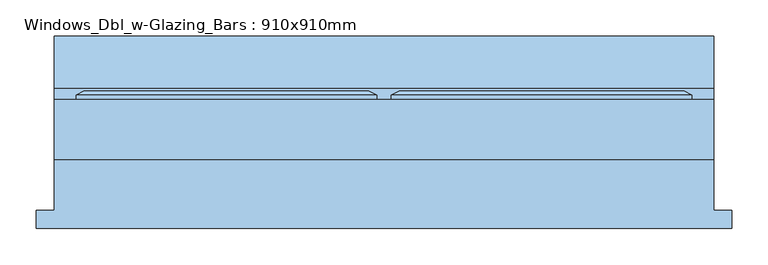
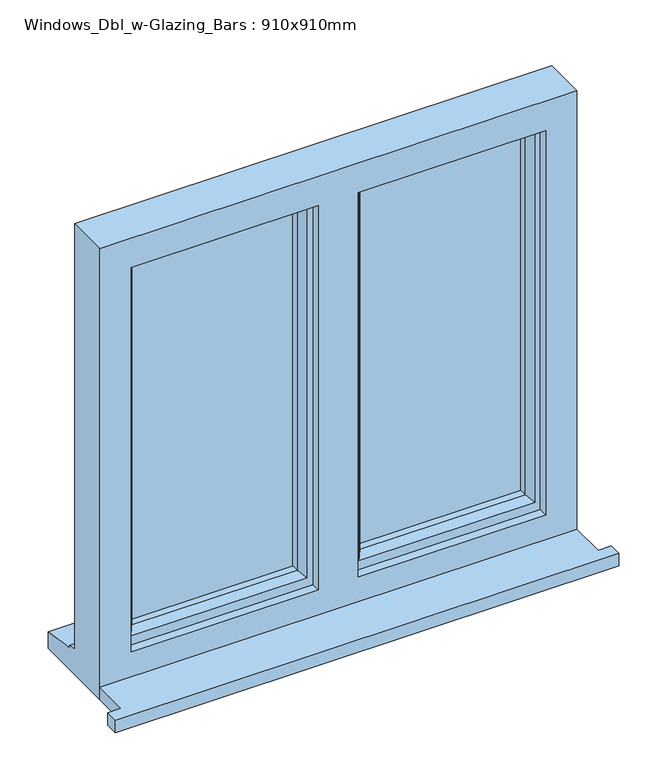
"""IFC4 building model written with IfcOpenShell, lengths in millimetres: window geometry, Windows_Dbl_w-Glazing_Bars : 910x910mm."""

from ifc_helpers import new_model, si_unit, frame, origin, place, context, project, spatial, polyline, outline, extrude, faceted_brep, source, transform, mapped, element, save


def windows_dbl_w_glazing_bars_910x910mm_41eba874(model_context):
    return source(origin(), model_context, "Body", "SolidModel", [
        extrude(outline(polyline([(-610.0, -118.1434322), (-610.0, -93.1434322), (-585.0, -93.1434322), (-585.0, -22.9434322), (325.0, -22.9434322), (325.0, -93.1434322), (350.0, -93.1434322), (350.0, -118.1434322), (-610.0, -118.1434322)])), frame((0.0, 0.0, 1190.0), z_axis=(0.0, 0.0, 1.0), x_axis=(1.0, 0.0, 0.0)), (0.0, 0.0, 1.0), 25.0),
        faceted_brep([(-120.0, 60.0565678, 2070.0), (-120.0, 65.8300705, 2070.0), (-120.0, 65.8300705, 1243.0), (-120.0, 60.0565678, 1243.0), (-110.0, -4.9434322, 2060.0), (-110.0, 60.0565678, 2060.0), (-110.0, 60.0565678, 1253.0), (-110.0, -4.9434322, 1253.0), (-70.0, 9.5494677, 2020.0), (-80.1480377, -4.9434322, 2030.1480377), (-80.1480377, -4.9434322, 1282.8519623), (-70.0, 9.5494677, 1293.0), (-70.0, 24.0565678, 2020.0), (-70.0, 24.0565678, 1293.0), (-80.0, 48.0565678, 2030.0), (-80.0, 24.0565678, 2030.0), (-80.0, 24.0565678, 1283.0), (-80.0, 48.0565678, 1283.0), (-70.0, 65.8300705, 2020.0), (-70.0, 48.0565678, 2020.0), (-70.0, 48.0565678, 1293.0), (-70.0, 65.8300705, 1293.0), (-87.4457548, 71.6035732, 2037.4457548), (-87.4457548, 71.6035732, 1275.5542452), (-109.2153903, 71.6035732, 2059.2153903), (-109.2153903, 71.6035732, 1253.7846097), (295.0, 65.8300705, 1243.0), (295.0, 60.0565678, 1243.0), (285.0, 60.0565678, 1253.0), (285.0, -4.9434322, 1253.0), (255.1480377, -4.9434322, 1282.8519623), (245.0, 9.5494677, 1293.0), (245.0, 24.0565678, 1293.0), (255.0, 24.0565678, 1283.0), (255.0, 48.0565678, 1283.0), (245.0, 48.0565678, 1293.0), (245.0, 65.8300705, 1293.0), (262.4457548, 71.6035732, 1275.5542452), (284.2153903, 71.6035732, 1253.7846097), (295.0, 65.8300705, 2070.0), (295.0, 60.0565678, 2070.0), (285.0, 60.0565678, 2060.0), (285.0, -4.9434322, 2060.0), (255.1480377, -4.9434322, 2030.1480377), (245.0, 9.5494677, 2020.0), (245.0, 24.0565678, 2020.0), (255.0, 24.0565678, 2030.0), (255.0, 48.0565678, 2030.0), (245.0, 48.0565678, 2020.0), (245.0, 65.8300705, 2020.0), (262.4457548, 71.6035732, 2037.4457548), (284.2153903, 71.6035732, 2059.2153903)], [[[0, 1, 2, 3]], [[4, 5, 6, 7]], [[8, 9, 10, 11]], [[12, 8, 11, 13]], [[14, 15, 16, 17]], [[18, 19, 20, 21]], [[22, 18, 21, 23]], [[1, 24, 25, 2]], [[3, 2, 26, 27]], [[7, 6, 28, 29]], [[11, 10, 30, 31]], [[13, 11, 31, 32]], [[17, 16, 33, 34]], [[21, 20, 35, 36]], [[23, 21, 36, 37]], [[2, 25, 38, 26]], [[27, 26, 39, 40]], [[29, 28, 41, 42]], [[31, 30, 43, 44]], [[32, 31, 44, 45]], [[34, 33, 46, 47]], [[36, 35, 48, 49]], [[37, 36, 49, 50]], [[26, 38, 51, 39]], [[40, 39, 1, 0]], [[3, 27, 40, 0], [5, 41, 28, 6]], [[42, 41, 5, 4]], [[7, 29, 42, 4], [9, 43, 30, 10]], [[44, 43, 9, 8]], [[45, 44, 8, 12]], [[15, 46, 33, 16], [13, 32, 45, 12]], [[47, 46, 15, 14]], [[17, 34, 47, 14], [19, 48, 35, 20]], [[49, 48, 19, 18]], [[50, 49, 18, 22]], [[24, 51, 38, 25], [23, 37, 50, 22]], [[39, 51, 24, 1]]]),
        extrude(outline(polyline([(255.0, 24.0565678), (-80.0, 24.0565678), (-80.0, 48.0565678), (255.0, 48.0565678), (255.0, 24.0565678)])), frame((0.0, 0.0, 1283.0), z_axis=(0.0, 0.0, 1.0), x_axis=(1.0, 0.0, 0.0)), (0.0, 0.0, 1.0), 747.0),
        extrude(outline(polyline([(-180.0, 24.0565678), (-515.0, 24.0565678), (-515.0, 48.0565678), (-180.0, 48.0565678), (-180.0, 24.0565678)])), frame((0.0, 0.0, 1283.0), z_axis=(0.0, 0.0, 1.0), x_axis=(1.0, 0.0, 0.0)), (0.0, 0.0, 1.0), 747.0),
        faceted_brep([(-140.0, 60.0565678, 2070.0), (-140.0, 65.8300705, 2070.0), (-555.0, 65.8300705, 2070.0), (-555.0, 60.0565678, 2070.0), (-150.0, -4.9434322, 2060.0), (-150.0, 60.0565678, 2060.0), (-545.0, 60.0565678, 2060.0), (-545.0, -4.9434322, 2060.0), (-190.0, 9.5494677, 2020.0), (-179.8519623, -4.9434322, 2030.1480377), (-515.1480377, -4.9434322, 2030.1480377), (-505.0, 9.5494677, 2020.0), (-190.0, 24.0565678, 2020.0), (-505.0, 24.0565678, 2020.0), (-180.0, 48.0565678, 2030.0), (-180.0, 24.0565678, 2030.0), (-515.0, 24.0565678, 2030.0), (-515.0, 48.0565678, 2030.0), (-190.0, 65.8300705, 2020.0), (-190.0, 48.0565678, 2020.0), (-505.0, 48.0565678, 2020.0), (-505.0, 65.8300705, 2020.0), (-172.5542452, 71.6035732, 2037.4457548), (-522.4457548, 71.6035732, 2037.4457548), (-150.7846097, 71.6035732, 2059.2153903), (-544.2153903, 71.6035732, 2059.2153903), (-555.0, 65.8300705, 1243.0), (-555.0, 60.0565678, 1243.0), (-545.0, 60.0565678, 1253.0), (-545.0, -4.9434322, 1253.0), (-515.1480377, -4.9434322, 1282.8519623), (-505.0, 9.5494677, 1293.0), (-505.0, 24.0565678, 1293.0), (-515.0, 24.0565678, 1283.0), (-515.0, 48.0565678, 1283.0), (-505.0, 48.0565678, 1293.0), (-505.0, 65.8300705, 1293.0), (-522.4457548, 71.6035732, 1275.5542452), (-544.2153903, 71.6035732, 1253.7846097), (-140.0, 65.8300705, 1243.0), (-140.0, 60.0565678, 1243.0), (-150.0, 60.0565678, 1253.0), (-150.0, -4.9434322, 1253.0), (-179.8519623, -4.9434322, 1282.8519623), (-190.0, 9.5494677, 1293.0), (-190.0, 24.0565678, 1293.0), (-180.0, 24.0565678, 1283.0), (-180.0, 48.0565678, 1283.0), (-190.0, 48.0565678, 1293.0), (-190.0, 65.8300705, 1293.0), (-172.5542452, 71.6035732, 1275.5542452), (-150.7846097, 71.6035732, 1253.7846097)], [[[0, 1, 2, 3]], [[4, 5, 6, 7]], [[8, 9, 10, 11]], [[12, 8, 11, 13]], [[14, 15, 16, 17]], [[18, 19, 20, 21]], [[22, 18, 21, 23]], [[1, 24, 25, 2]], [[3, 2, 26, 27]], [[7, 6, 28, 29]], [[11, 10, 30, 31]], [[13, 11, 31, 32]], [[17, 16, 33, 34]], [[21, 20, 35, 36]], [[23, 21, 36, 37]], [[2, 25, 38, 26]], [[27, 26, 39, 40]], [[0, 3, 27, 40], [41, 28, 6, 5]], [[29, 28, 41, 42]], [[4, 7, 29, 42], [43, 30, 10, 9]], [[31, 30, 43, 44]], [[32, 31, 44, 45]], [[46, 33, 16, 15], [12, 13, 32, 45]], [[34, 33, 46, 47]], [[14, 17, 34, 47], [48, 35, 20, 19]], [[36, 35, 48, 49]], [[37, 36, 49, 50]], [[51, 38, 25, 24], [22, 23, 37, 50]], [[26, 38, 51, 39]], [[40, 39, 1, 0]], [[42, 41, 5, 4]], [[44, 43, 9, 8]], [[45, 44, 8, 12]], [[47, 46, 15, 14]], [[49, 48, 19, 18]], [[50, 49, 18, 22]], [[39, 51, 24, 1]]]),
        extrude(outline(polyline([(-80.1480377, 40.0565678), (255.0, 40.0565678), (255.0, 32.0565678), (-80.1480377, 32.0565678), (-80.1480377, 40.0565678)])), frame((0.0, 0.0, 1646.5), z_axis=(0.0, 0.0, 1.0), x_axis=(1.0, 0.0, 0.0)), (0.0, 0.0, 1.0), 20.0),
        extrude(outline(polyline([(-515.0, 40.0565678), (-180.0, 40.0565678), (-180.0, 32.0565678), (-515.0, 32.0565678), (-515.0, 40.0565678)])), frame((0.0, 0.0, 1646.5), z_axis=(0.0, 0.0, 1.0), x_axis=(1.0, 0.0, 0.0)), (0.0, 0.0, 1.0), 20.0),
        extrude(outline(polyline([(-80.1480377, 40.0565678), (255.0, 40.0565678), (255.0, 32.0565678), (-80.1480377, 32.0565678), (-80.1480377, 40.0565678)])), frame((0.0, 0.0, 1828.25), z_axis=(0.0, 0.0, 1.0), x_axis=(1.0, 0.0, 0.0)), (0.0, 0.0, 1.0), 20.0),
        extrude(outline(polyline([(-80.1480377, 40.0565678), (255.0, 40.0565678), (255.0, 32.0565678), (-80.1480377, 32.0565678), (-80.1480377, 40.0565678)])), frame((0.0, 0.0, 1464.75), z_axis=(0.0, 0.0, 1.0), x_axis=(1.0, 0.0, 0.0)), (0.0, 0.0, 1.0), 20.0),
        extrude(outline(polyline([(-515.0, 40.0565678), (-180.0, 40.0565678), (-180.0, 32.0565678), (-515.0, 32.0565678), (-515.0, 40.0565678)])), frame((0.0, 0.0, 1828.25), z_axis=(0.0, 0.0, 1.0), x_axis=(1.0, 0.0, 0.0)), (0.0, 0.0, 1.0), 20.0),
        extrude(outline(polyline([(-515.0, 40.0565678), (-180.0, 40.0565678), (-180.0, 32.0565678), (-515.0, 32.0565678), (-515.0, 40.0565678)])), frame((0.0, 0.0, 1464.75), z_axis=(0.0, 0.0, 1.0), x_axis=(1.0, 0.0, 0.0)), (0.0, 0.0, 1.0), 20.0),
        faceted_brep([(325.0, -22.9434322, 2100.0), (-585.0, -22.9434322, 2100.0), (-585.0, -22.9434322, 1190.0), (325.0, -22.9434322, 1190.0), (265.0, -22.9434322, 2040.0), (265.0, -22.9434322, 1265.0), (-92.0, -22.9434322, 1265.0), (-92.0, -22.9434322, 2040.0), (-168.0, -22.9434322, 2040.0), (-168.0, -22.9434322, 1265.0), (-525.0, -22.9434322, 1265.0), (-525.0, -22.9434322, 2040.0), (-585.0, 60.0565678, 2100.0), (-585.0, 60.0565678, 1241.0), (-585.0, 75.0565678, 1239.68767), (-585.0, 75.0565678, 1234.7449676), (-585.0, 147.5565678, 1223.8088847), (-585.0, 147.5565678, 1190.0), (325.0, 60.0565678, 2100.0), (325.0, 60.0565678, 1241.0), (-545.0, 60.0565678, 2060.0), (-545.0, 60.0565678, 1253.0), (-150.0, 60.0565678, 1253.0), (-150.0, 60.0565678, 2060.0), (-110.0, 60.0565678, 2060.0), (-110.0, 60.0565678, 1253.0), (285.0, 60.0565678, 1253.0), (285.0, 60.0565678, 2060.0), (-545.0, -4.9434322, 2060.0), (-545.0, -4.9434322, 1253.0), (-150.0, -4.9434322, 2060.0), (-150.0, -4.9434322, 1253.0), (-168.0, -4.9434322, 2040.0), (-525.0, -4.9434322, 2040.0), (-525.0, -4.9434322, 1265.0), (-168.0, -4.9434322, 1265.0), (-110.0, -4.9434322, 2060.0), (285.0, -4.9434322, 2060.0), (285.0, -4.9434322, 1253.0), (-110.0, -4.9434322, 1253.0), (265.0, -4.9434322, 2040.0), (-92.0, -4.9434322, 2040.0), (-92.0, -4.9434322, 1265.0), (265.0, -4.9434322, 1265.0), (325.0, 147.5565678, 1190.0), (325.0, 147.5565678, 1223.8088847), (325.0, 75.0565678, 1234.7449676), (325.0, 75.0565678, 1239.68767)], [[[0, 1, 2, 3], [4, 5, 6, 7], [8, 9, 10, 11]], [[2, 1, 12, 13, 14, 15, 16, 17]], [[13, 12, 18, 19], [20, 21, 22, 23], [24, 25, 26, 27]], [[21, 20, 28, 29]], [[28, 30, 31, 29], [32, 33, 34, 35]], [[36, 37, 38, 39], [40, 41, 42, 43]], [[33, 11, 10, 34]], [[1, 0, 18, 12]], [[28, 20, 23, 30]], [[27, 37, 36, 24]], [[11, 33, 32, 8]], [[40, 4, 7, 41]], [[19, 18, 0, 3, 44, 45, 46, 47]], [[27, 26, 38, 37]], [[4, 40, 43, 5]], [[41, 7, 6, 42]], [[8, 32, 35, 9]], [[23, 22, 31, 30]], [[25, 24, 36, 39]], [[44, 3, 2, 17]], [[45, 44, 17, 16]], [[46, 45, 16, 15]], [[47, 46, 15, 14]], [[19, 47, 14, 13]], [[22, 21, 29, 31]], [[39, 38, 26, 25]], [[6, 5, 43, 42]], [[35, 34, 10, 9]]]),
    ])


if __name__ == "__main__":
    model = new_model("IFC4")
    model_context = context("Model", 3, world=origin())
    ifc_project = project(units=[si_unit("LENGTHUNIT", "METRE", prefix="MILLI")], contexts=[model_context])
    site = spatial("IfcSite", under=ifc_project)
    building = spatial("IfcBuilding", under=site)
    placement = place(None, origin())
    windows_dbl_w_glazing_bars_910x910mm_shape = windows_dbl_w_glazing_bars_910x910mm_41eba874(model_context)
    element("IfcWindow", 1, ObjectType="Windows_Dbl_w-Glazing_Bars : 910x910mm", at=placement, inside=building, context=model_context, shape_type="MappedRepresentation", body=[
        mapped(windows_dbl_w_glazing_bars_910x910mm_shape, transform((0.0, 0.0, 0.0), x_axis=(1.0, 0.0, 0.0), y_axis=(0.0, 1.0, 0.0), z_axis=(0.0, 0.0, 1.0))),
    ])
    save(model, "model.ifc")

# Revit data of these elements
# Type "Windows_Dbl_w-Glazing_Bars : 910x910mm"
#   Type Mark = "33"
#   Operation = "DoublePanelVertical"
#   Construction Type Id = "GSP4R"
#   Manufacturer = "Revit"
#   Keynote = "L10"
#   Analytic Construction = "1/8 in Pilkington single glazing"
#   Wrap Layers (Ext) from Ext = 0' - 4.03543"
#   Wrap Layers (Int) from Ext = 0' - 6.98819"
#   Window Board Projection = 0' - 0.98425"
#   Window Board Extension = 0' - 0.98425"
#   Visual Light Transmittance = 0.9
#   Solar Heat Gain Coefficient = 0.78
#   Rough Width = 2' - 11.82677"
#   Rough Height = 2' - 11.82677"
#   Height = 2' - 11.82677"
#   Width = 2' - 11.82677"
#   Heat Transfer Coefficient (U) = 0.6496 BTU/(h·ft²·°F)
#   Glazing Thickness = 0' - 0.94488"
#   Glazing Bar Thickness = 0' - 0.7874"
#   FrameOffset - External = 0' - 1.9685"
#   Frame Depth = 0' - 2.55906"
#   Default Head Height = 6' - 10.67717"
#   Cill Depth = 0' - 3.44488"
#   Cavity Closer Width = 0' - 1.9685"
#   Cavity Closer Offset from Ext = 0' - 4.03543"
#   Cavity Closer Depth = 0' - 3.34646"
#   Vis - Glazing Bars = yes
#   Vis - Cavity Closers = yes
#   Define Thermal Properties by = 1
#   Material Trim = Window Frame
#   Material Glazing Bars = Window Frame
#   Material Glass = Glass
#   Material Frame = Window Frame
#   Wall Closure = (empty or 0)
# Element 1 (IfcWindow, "Windows_Dbl_w-Glazing_Bars : 910x910mm")
#   Materials on its faces: "Window Frame", "Glass"
# Materials
#   "Window Frame": colour RGB 249 249 249, transparency 0
#   "Glass": class "Glass", colour RGB 0 128 192, transparency 0.75, Description = "Soda Lime Glass", Cost = 0
